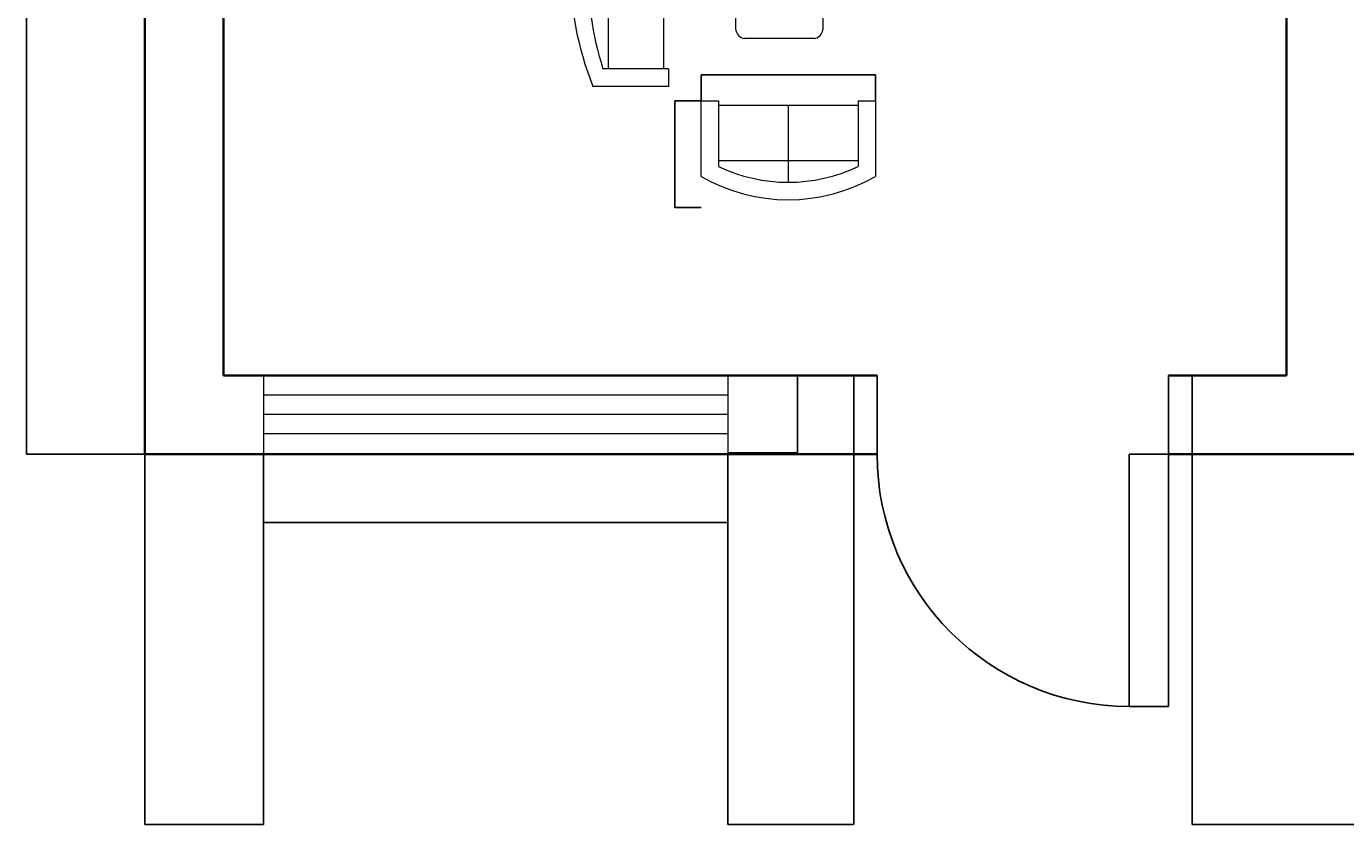
# Model space of a CAD drawing. Units: millimetres. Extents: x 726 to 37095, y -1634 to 13537.
# Tile 1 of 4: x 726 to 9102, y -1568 to 3500. Entities that reach past the tile are written whole.
import ezdxf

# ---------------------------------------------------------------- set-up
doc = ezdxf.new("R2010")
doc.units = ezdxf.units.MM
for name, color, linetype, lineweight in [('A-ANNO-DIMS', 2, 'Continuous', 18), ('A-DOOR', 3, 'Continuous', 25), ('A-FURN', 8, 'Continuous', 18), ('A-GLAZ', 4, 'Continuous', 18), ('A-WALL', 7, 'Continuous', 35)]:
    doc.layers.add(name, color=color, linetype=linetype, lineweight=lineweight)
doc.styles.get("Standard").update_dxf_attribs({"font": 'arial.ttf'})
doc.dimstyles.get("Standard").update_dxf_attribs({"dimtxt": 0.18, "dimasz": 0.18, "dimexe": 0.18, "dimexo": 0.0625, "dimgap": 0.09, "dimtad": 0, "dimtih": 1, "dimtoh": 1, "dimdec": 4, "dimzin": 0, "dimdsep": 46, "dimtxsty": 'Standard', "dimcen": 0.09, "dimadec": 0, "dimazin": 0, "dimtfac": 1, "dimtdec": 4, "dimtofl": 0, "dimtmove": 0, "dimatfit": 3, "dimfxl": 1, "dimtolj": 1, "dimtzin": 0, "dimarcsym": 0})

# ---------------------------------------------------------------- blocks, each defined once
blk = doc.blocks.new('Sofa - Roundback 7 ft.')
for p, q in [((-12.00002, -32.44210000000393), (-12.00003, -6.597100000003898)), ((11.99996999999999, -32.44210000000393), (11.99997999999999, -6.597100000003898)), ((-36.000027, -34.00000000000395), (-36.000027, -11.46960000000396)), ((-35.999844, -13.38190000000397), (35.99979999999999, -13.38190000000397)), ((35.99997999999999, -34.00000000000395), (35.99997999999999, -11.46960000000396)), ((-36.000027, -32.44210000000393), (35.99997999999999, -32.44210000000393))]:
    blk.add_line(p, q)
for points in [[(-36.000027, -34.00000000000395), (-42.000027, -34.00000000000395), (-42.000027, -8.000000000003944)], [(41.99997999999999, -8.000000000003944), (41.99997999999999, -34.00000000000395), (35.99997999999999, -34.00000000000395)]]:
    blk.add_lwpolyline(points)
for centre, radius, start, end in [((0, -114.2500000000039), 114.2500000000039, 68.43141000000072, 111.5686000000006), ((-1.00000000032e-05, -127.1968000000039), 121.1967999999973, 72.72032999999948, 107.2797000000005)]:
    blk.add_arc(centre, radius, start, end)
blk = doc.blocks.new('Sofa - Roundback Loveseat 5 ft.')
for p, q in [((0, -32.44198000000246), (0, -5.999980000002448)), ((-23.99999999999999, -33.99998000000245), (-23.99999999999999, -11.46958000000243)), ((-23.99979999999998, -13.38178000000245), (23.99986, -13.38178000000245)), ((24.00004000000001, -33.99998000000245), (24.00004000000001, -11.46958000000243)), ((-23.99999999999999, -32.44198000000246), (24.00004000000001, -32.44198000000246))]:
    blk.add_line(p, q)
for points in [[(-23.99999999999999, -33.99998000000245), (-29.99999999999999, -33.99998000000245), (-29.99999999999999, -7.999980000002448)], [(30.00004000000001, -7.999980000002448), (30.00004000000001, -33.99998000000245), (24.00004000000001, -33.99998000000245)]]:
    blk.add_lwpolyline(points)
for centre, radius, start, end in [((0, -60.24998000000245), 60.24998000000245, 60.13715000000122, 119.862800000004), ((0, -61.38438000000245), 55.38444000000723, 64.32083000000306, 115.6791999999996)]:
    blk.add_arc(centre, radius, start, end)
blk = doc.blocks.new('Desk - 30 x 60 in.')
for p, q in [((-26.999995, 0), (26.999995, 0)), ((-29.999995, -27), (-29.999995, -3)), ((29.999995, -3), (29.999995, -27)), ((26.999995, -30), (-26.999995, -30)), ((-20.000005, -30), (-20.000005, -31)), ((-20.000005, -31), (-16.000005, -31)), ((-16.000005, -31), (-16.000005, -30)), ((15.999995, -31), (15.999995, -30)), ((19.999995, -31), (15.999995, -31)), ((19.999995, -30), (19.999995, -31))]:
    blk.add_line(p, q)
for centre, radius, start, end in [((-26.499995, -3.5), 3.535534000004229, 98.1300999999916, 171.8698999999352), ((26.499995, -3.5), 3.535533999997753, 8.130102000022115, 81.8698999999439), ((-26.499995, -26.5), 3.535534000000845, 188.1301000000653, 261.8699000000085), ((26.499995, -26.5), 3.535534000004826, 278.1301000000561, 351.8698999999439)]:
    blk.add_arc(centre, radius, start, end)
blk = doc.blocks.new('Window - Wood Frame 36 in. Wide plan')
for p, q in [((0, 6), (0, 0)), ((36, 6), (36, 0)), ((0, 4.5), (36, 4.5)), ((0, 3), (36, 3)), ((0, 1.5), (36, 1.5))]:
    blk.add_line(p, q)
blk = doc.blocks.new('DOOR-ENTRY-1601')
for p, q in [((0, 1600.959499914892), (0, 2101.259343638296)), ((0, 2101.259343638296), (148.488993617113, 2101.259343638296)), ((148.488993617113, 2101.259343638296), (148.488993617113, 1600.959499914892)), ((1999.598415393706, 1600.959499914892), (1999.598415393706, 2101.259343638296)), ((1999.598415393706, 2101.259343638296), (2148.087409010808, 2101.259343638296)), ((2148.087409010808, 2101.259343638296), (2148.087409010808, 1600.959499914892)), ((148.488993617113, 1600.959499914892), (0, 1600.959499914892)), ((148.488993617113, 1600.959499914892), (148.488993617113, -1.137e-13)), ((398.6389154788158, 1600.959499914892), (148.488993617113, 1600.959499914892)), ((148.488993617113, 1600.959499914892), (398.6389154788158, 1600.959499914892)), ((398.6389154788158, 1600.959499914892), (398.6389154788158, -1.137e-13)), ((2148.087409010808, 1600.959499914892), (1999.598415393706, 1600.959499914892)), ((148.488993617113, -1.137e-13), (398.6389154788158, -1.137e-13))]:
    blk.add_line(p, q)
blk.add_arc((398.6389154788158, 1600.959499914892), 1600.959499914892, 270, 0)
blk = doc.blocks.new('*D15')
at = {"layer": 'A-ANNO-DIMS', "color": 0, "lineweight": -2, "transparency": 16777216}
for p, q in [((2231.692889473896, 792.4362370827457), (2231.692889473896, 350.0703191466211)), ((5180.015675714727, 792.4362370827457), (5180.015675714727, 350.0703191466211)), ((2231.872889473896, 350.2503191466211), (3704.087556809864, 350.2503191466211)), ((5179.835675714727, 350.2503191466211), (3707.621008378759, 350.2503191466211))]:
    blk.add_line(p, q, dxfattribs=at)
at = {"layer": 'A-ANNO-DIMS', "color": 0, "transparency": 16777216}
for points in [[(2231.872889473896, 350.280319146621), (2231.872889473896, 350.2203191466211), (2231.692889473896, 350.2503191466211)], [(5179.835675714727, 350.280319146621), (5179.835675714727, 350.2203191466211), (5180.015675714727, 350.2503191466211)]]:
    blk.add_solid(points, dxfattribs=at)
at = {"layer": 'Defpoints', "color": 0, "transparency": 16777216}
for p in [(2231.692889473896, 792.4987370827457), (5180.015675714727, 792.4987370827457), (5180.015675714727, 350.2503191466211)]:
    blk.add_point(p, dxfattribs=at)
at = {"layer": 'A-ANNO-DIMS', "color": 0, "transparency": 16777216, "insert": (3705.854282594311, 350.2503191466211), "char_height": 0.18, "attachment_point": 5}
blk.add_mtext('\\A1;TIMBER WINDOW 2948 TYP.', dxfattribs=at)
blk = doc.blocks.new('*D16')
at = {"layer": 'A-ANNO-DIMS', "color": 0, "lineweight": -2, "transparency": 16777216}
for p, q in [((5180.078175714729, 1283.885868122884), (5622.444093650855, 1283.885868122884)), ((5622.264093650855, 1283.705868122885), (5622.264093650855, 1038.374205740605)), ((5622.264093650855, 792.6787370827462), (5622.264093650855, 1038.010399465025)), ((5180.078175714729, 792.4987370827461), (5622.444093650855, 792.4987370827462))]:
    blk.add_line(p, q, dxfattribs=at)
at = {"layer": 'A-ANNO-DIMS', "color": 0, "transparency": 16777216}
for points in [[(5622.234093650855, 1283.705868122885), (5622.294093650855, 1283.705868122885), (5622.264093650855, 1283.885868122884)], [(5622.234093650855, 792.6787370827462), (5622.294093650855, 792.6787370827462), (5622.264093650855, 792.4987370827462)]]:
    blk.add_solid(points, dxfattribs=at)
at = {"layer": 'Defpoints', "color": 0, "transparency": 16777216}
for p in [(5180.015675714729, 1283.885868122884), (5622.264093650855, 1283.885868122884), (5180.015675714729, 792.4987370827461)]:
    blk.add_point(p, dxfattribs=at)
at = {"layer": 'A-ANNO-DIMS', "color": 0, "transparency": 16777216, "insert": (5622.264093650854, 1038.192302602813), "char_height": 0.18, "attachment_point": 5}
blk.add_mtext('\\A1;491 TYP.', dxfattribs=at)
blk = doc.blocks.new('*D27')
at = {"layer": 'A-ANNO-DIMS', "color": 0, "lineweight": -2, "transparency": 16777216}
for p, q in [((5009.763478172475, 3027.085310713908), (5009.763478172475, 3193.347378938926)), ((5009.943478172475, 3193.167378938926), (5562.21599754009, 3193.167378938926)), ((6117.213933005931, 3193.167378938926), (5564.941413638316, 3193.167378938926)), ((6117.393933005931, 3027.085310713907), (6117.393933005931, 3193.347378938926))]:
    blk.add_line(p, q, dxfattribs=at)
at = {"layer": 'A-ANNO-DIMS', "color": 0, "transparency": 16777216}
for points in [[(5009.943478172475, 3193.197378938926), (5009.943478172475, 3193.137378938926), (5009.763478172475, 3193.167378938926)], [(6117.213933005931, 3193.197378938926), (6117.213933005931, 3193.137378938926), (6117.393933005931, 3193.167378938926)]]:
    blk.add_solid(points, dxfattribs=at)
at = {"layer": 'Defpoints', "color": 0, "transparency": 16777216}
for p in [(5009.763478172475, 3193.167378938926), (5009.763478172475, 3027.022810713908), (6117.393933005931, 3027.022810713908)]:
    blk.add_point(p, dxfattribs=at)
at = {"layer": 'A-ANNO-DIMS', "color": 0, "transparency": 16777216, "insert": (5563.578705589203, 3193.167378938926), "char_height": 0.18, "attachment_point": 5}
blk.add_mtext('\\A1;LOVESEAT 1108 TYP.', dxfattribs=at)
blk = doc.blocks.new('*D28')
at = {"layer": 'A-ANNO-DIMS', "color": 0, "lineweight": -2, "transparency": 16777216}
for p, q in [((5009.700978172476, 3027.022810713909), (4843.438909947459, 3027.022810713909)), ((4843.618909947459, 3026.842810713909), (4843.618909947459, 2688.76246234902)), ((4843.618909947459, 2350.31830770855), (4843.618909947459, 2688.39865607344)), ((5009.700978172476, 2350.13830770855), (4843.438909947459, 2350.13830770855))]:
    blk.add_line(p, q, dxfattribs=at)
at = {"layer": 'A-ANNO-DIMS', "color": 0, "transparency": 16777216}
for points in [[(4843.58890994746, 3026.842810713909), (4843.648909947459, 3026.842810713909), (4843.618909947459, 3027.022810713909)], [(4843.58890994746, 2350.31830770855), (4843.648909947459, 2350.31830770855), (4843.618909947459, 2350.13830770855)]]:
    blk.add_solid(points, dxfattribs=at)
at = {"layer": 'Defpoints', "color": 0, "transparency": 16777216}
for p in [(5009.763478172477, 3027.022810713909), (4843.618909947459, 2350.13830770855), (5009.763478172477, 2350.13830770855)]:
    blk.add_point(p, dxfattribs=at)
at = {"layer": 'A-ANNO-DIMS', "color": 0, "transparency": 16777216, "insert": (4843.618909947459, 2688.580559211228), "char_height": 0.18, "attachment_point": 5}
blk.add_mtext('\\A1;677 TYP.', dxfattribs=at)
blk = doc.blocks.new('*D44')
at = {"layer": 'A-ANNO-DIMS', "color": 0, "lineweight": -2, "transparency": 16777216}
for p, q in [((1477.247346, 12783.885868), (726.3798459999991, 12783.885868)), ((726.559845999999, 12783.705868), (726.5598460000004, 6784.067771137793)), ((726.5598460000017, 784.0658680000001), (726.5598460000004, 6783.703964862214)), ((1477.247346, 783.8858680000003), (726.3798460000017, 783.8858680000002))]:
    blk.add_line(p, q, dxfattribs=at)
at = {"layer": 'A-ANNO-DIMS', "color": 0, "transparency": 16777216}
for points in [[(726.5298459999991, 12783.705868), (726.589845999999, 12783.705868), (726.559845999999, 12783.885868)], [(726.5298460000017, 784.0658680000001), (726.5898460000016, 784.0658680000001), (726.5598460000017, 783.8858680000002)]]:
    blk.add_solid(points, dxfattribs=at)
at = {"layer": 'Defpoints', "color": 0, "transparency": 16777216}
for p in [(726.559845999999, 12783.885868), (1477.309846, 12783.885868), (1477.309846, 783.8858680000003)]:
    blk.add_point(p, dxfattribs=at)
at = {"layer": 'A-ANNO-DIMS', "color": 0, "transparency": 16777216, "insert": (726.5598460000022, 6783.885868000002), "char_height": 0.18, "attachment_point": 5}
blk.add_mtext('\\A1;12000', dxfattribs=at)
blk = doc.blocks.new('*D57')
at = {"layer": 'A-ANNO-DIMS', "color": 0, "lineweight": -2, "transparency": 16777216}
for p, q in [((1477.309846, 783.823368), (1477.309846, -1568.303476)), ((2231.692889, 792.4362369999999), (2231.692889, -1568.303476)), ((1477.489846, -1568.123476), (1854.108768591405, -1568.123476)), ((2231.512889, -1568.123476), (1854.893966408595, -1568.123476))]:
    blk.add_line(p, q, dxfattribs=at)
at = {"layer": 'A-ANNO-DIMS', "color": 0, "transparency": 16777216}
for points in [[(1477.489846, -1568.093476), (1477.489846, -1568.153476), (1477.309846, -1568.123476)], [(2231.512889, -1568.093476), (2231.512889, -1568.153476), (2231.692889, -1568.123476)]]:
    blk.add_solid(points, dxfattribs=at)
at = {"layer": 'Defpoints', "color": 0, "transparency": 16777216}
for p in [(1477.309846, 783.8858679999998), (2231.692889, 792.498737), (2231.692889, -1568.123476)]:
    blk.add_point(p, dxfattribs=at)
at = {"layer": 'A-ANNO-DIMS', "color": 0, "transparency": 16777216, "insert": (1854.5013675, -1568.123476), "char_height": 0.18, "attachment_point": 5}
blk.add_mtext('\\A1;754.4', dxfattribs=at)
blk = doc.blocks.new('*D58')
at = {"layer": 'A-ANNO-DIMS', "color": 0, "lineweight": -2, "transparency": 16777216}
for p, q in [((5180.015676, 792.4362369999999), (5180.015676, -1568.303476)), ((5978.976829, 783.523524), (5978.976829, -1568.303476)), ((5180.195676, -1568.123476), (5579.2079578206, -1568.123476)), ((5978.796829, -1568.123476), (5579.7845471794, -1568.123476))]:
    blk.add_line(p, q, dxfattribs=at)
at = {"layer": 'A-ANNO-DIMS', "color": 0, "transparency": 16777216}
for points in [[(5180.195676, -1568.093476), (5180.195676, -1568.153476), (5180.015676, -1568.123476)], [(5978.796829, -1568.093476), (5978.796829, -1568.153476), (5978.976829, -1568.123476)]]:
    blk.add_solid(points, dxfattribs=at)
at = {"layer": 'Defpoints', "color": 0, "transparency": 16777216}
for p in [(5180.015676, 792.498737), (5978.976829, 783.586024), (5978.976829, -1568.123476)]:
    blk.add_point(p, dxfattribs=at)
at = {"layer": 'A-ANNO-DIMS', "color": 0, "transparency": 16777216, "insert": (5579.4962525, -1568.123476), "char_height": 0.18, "attachment_point": 5}
blk.add_mtext('\\A1;799', dxfattribs=at)
blk = doc.blocks.new('*D59')
at = {"layer": 'A-ANNO-DIMS', "color": 0, "lineweight": -2, "transparency": 16777216}
for p, q in [((8127.064238, 783.523524), (8127.064238, -1568.303476)), ((9695.60409, 783.523524), (9695.60409, -1568.303476)), ((8127.244238000001, -1568.123476), (8910.878331803548, -1568.123476)), ((9695.42409, -1568.123476), (8911.789996196452, -1568.123476))]:
    blk.add_line(p, q, dxfattribs=at)
at = {"layer": 'A-ANNO-DIMS', "color": 0, "transparency": 16777216}
for points in [[(8127.244238000001, -1568.093476), (8127.244238000001, -1568.153476), (8127.064238, -1568.123476)], [(9695.42409, -1568.093476), (9695.42409, -1568.153476), (9695.60409, -1568.123476)]]:
    blk.add_solid(points, dxfattribs=at)
at = {"layer": 'Defpoints', "color": 0, "transparency": 16777216}
for p in [(8127.064238, 783.586024), (9695.60409, 783.586024), (9695.60409, -1568.123476)]:
    blk.add_point(p, dxfattribs=at)
at = {"layer": 'A-ANNO-DIMS', "color": 0, "transparency": 16777216, "insert": (8911.334164000002, -1568.123476), "char_height": 0.18, "attachment_point": 5}
blk.add_mtext('\\A1;1568.5', dxfattribs=at)

msp = doc.modelspace()

# ---------------------------------------------------------------- linework, layer by layer
at = {"layer": 'A-WALL'}
for p, q in [((1477.309845865288, 12783.88586812288), (1477.309845865288, 783.8858681228857)), ((1977.309845865287, 8533.885868122883), (1977.309845865287, 1283.885868122886)), ((8727.30984586529, 8534.561644066505), (8727.309845865288, 1283.885868122885)), ((1977.309845865287, 1283.885868122886), (6127.465822806607, 1283.885868122886)), ((7978.5752445832, 1283.885868122886), (8727.309845865286, 1283.885868122885)), ((1477.309845865288, 783.8858681228857), (6127.465822806607, 783.8858681228859)), ((7978.5752445832, 783.8858681228859), (9844.093083592761, 783.8858681228859))]:
    msp.add_line(p, q, dxfattribs=at)

# ---------------------------------------------------------------- block references
at = {"layer": 'A-DOOR', "extrusion": (0, 0, -1), "zscale": -1}
msp.add_blockref('DOOR-ENTRY-1601', (-8127.064238200311, -817.3734755154111), dxfattribs=at)
at = {"layer": 'A-FURN', "xscale": 18.46049527356076, "yscale": 18.46049527356076, "zscale": 18.46049527356076}
for name, p, rotation in [('Sofa - Roundback 7 ft.', (4175.152231439681, 3894.653569822566), 90), ('Desk - 30 x 60 in.', (5229.86281300102, 3977.274990980613), 90), ('Sofa - Roundback Loveseat 5 ft.', (5563.579074799109, 2399.366340622702), 180)]:
    msp.add_blockref(name, p, dxfattribs=dict(at, rotation=rotation))
at = {"layer": 'A-GLAZ', "xscale": 81.8978551733564, "yscale": 81.8978551733564, "zscale": 81.8978551733564}
msp.add_blockref('Window - Wood Frame 36 in. Wide plan', (2231.692889473896, 792.4987370827457), dxfattribs=at)

# ---------------------------------------------------------------- dimensions: what is measured, and where the dimension line sits
at = {"layer": 'A-ANNO-DIMS'}
dim = msp.add_linear_dim(base=(726.559845999999, 12783.885868), p1=(1477.309846, 783.8858679999998), p2=(1477.309846, 12783.885868), angle=90, dimstyle='Standard', override={"dimdec": 0, "dimlfac": 1, "dimrnd": 0, "dimzin": 0, "dimdsep": 46, "dimlunit": 2}, dxfattribs=at)
dim.commit()
dim.dimension.update_dxf_attribs({"geometry": '*D44', "text_midpoint": (726.5598460000022, 6783.885868000002)})
for base, p1, p2, angle, text, picture, middle in [((5009.763478172475, 3193.167378938926), (6117.393933005931, 3027.022810713908), (5009.763478172475, 3027.022810713908), 180, 'LOVESEAT <> TYP.', '*D27', (5563.578705589203, 3193.167378938926)), ((4843.618909947459, 2350.13830770855), (5009.763478172475, 3027.022810713908), (5009.763478172475, 2350.138307708549), 270, '<> TYP.', '*D28', (4843.618909947459, 2688.580559211228)), ((5622.264093650855, 1283.885868122884), (5180.015675714727, 792.4987370827457), (5180.015675714727, 1283.885868122884), 90, '<> TYP.', '*D16', (5622.264093650854, 1038.192302602813))]:
    dim = msp.add_linear_dim(base=base, p1=p1, p2=p2, angle=angle, text=text, dimstyle='Standard', override={"dimdec": 0, "dimlfac": 1, "dimrnd": 0, "dimzin": 0, "dimdsep": 46, "dimlunit": 2}, dxfattribs=at)
    dim.commit()
    dim.dimension.update_dxf_attribs({"geometry": picture, "text_midpoint": middle})
for base, p1, p2, override, picture, middle in [((2231.692889, -1568.123476), (1477.309846, 783.8858679999998), (2231.692889, 792.498737), {"dimdec": 1, "dimlfac": 1, "dimrnd": 0, "dimzin": 0, "dimdsep": 46, "dimlunit": 2}, '*D57', (1854.5013675, -1568.123476)), ((5978.976829, -1568.123476), (5180.015676, 792.498737), (5978.976829, 783.586024), {"dimdec": 0, "dimlfac": 1, "dimrnd": 0, "dimzin": 0, "dimdsep": 46, "dimlunit": 2}, '*D58', (5579.4962525, -1568.123476)), ((9695.60409, -1568.123476), (8127.064238, 783.586024), (9695.60409, 783.586024), {"dimdec": 1, "dimlfac": 1, "dimrnd": 0, "dimzin": 0, "dimdsep": 46, "dimlunit": 2}, '*D59', (8911.334164000002, -1568.123476))]:
    dim = msp.add_linear_dim(base=base, p1=p1, p2=p2, dimstyle='Standard', override=override, dxfattribs=at)
    dim.commit()
    dim.dimension.update_dxf_attribs({"geometry": picture, "text_midpoint": middle})
dim = msp.add_linear_dim(base=(5180.015675714727, 350.2503191466211), p1=(2231.692889473896, 792.4987370827457), p2=(5180.015675714727, 792.4987370827457), text='TIMBER WINDOW <> TYP.', dimstyle='Standard', override={"dimdec": 0, "dimlfac": 1, "dimrnd": 0, "dimzin": 0, "dimdsep": 46, "dimlunit": 2}, dxfattribs=at)
dim.commit()
dim.dimension.update_dxf_attribs({"geometry": '*D15', "text_midpoint": (3705.854282594311, 350.2503191466211)})

doc.saveas('drawing.dxf')
